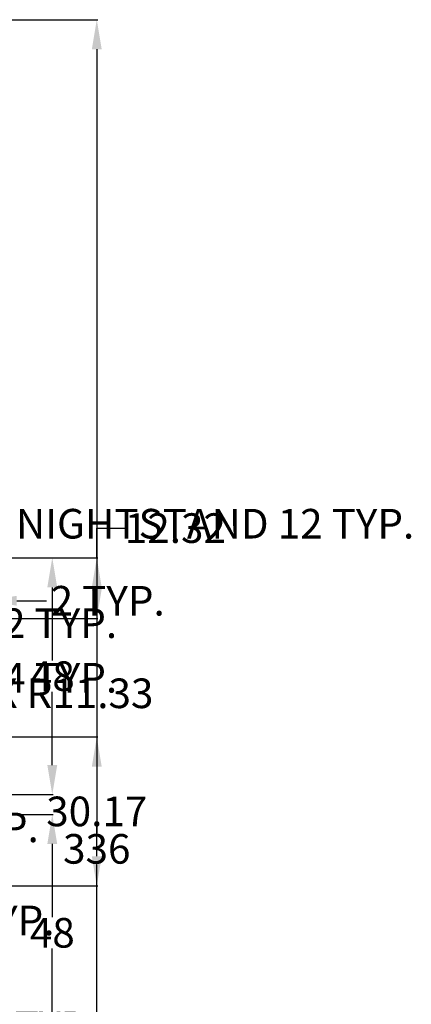
# Model space of a CAD drawing. Units: inches. Extents: x 98 to 487, y -240 to 141.
# Tile 5 of 5: x 408 to 487, y -81 to 119. Entities that reach past the tile are written whole.
import ezdxf

# ---------------------------------------------------------------- set-up
doc = ezdxf.new("R2010")
doc.units = ezdxf.units.IN
doc.header["$MEASUREMENT"] = 0
doc.layers.add('A-ANNO-DIMS', color=2, linetype='Continuous', lineweight=18)
doc.styles.get("Standard").update_dxf_attribs({"font": 'arial.ttf'})
doc.dimstyles.get("Standard").update_dxf_attribs({"dimtxt": 6, "dimasz": 6, "dimexe": 0.18, "dimexo": 0.0625, "dimgap": 0.09, "dimtad": 0, "dimtih": 1, "dimtoh": 1, "dimdec": 0, "dimzin": 0, "dimdsep": 46, "dimlunit": 4, "dimtxsty": 'Standard', "dimcen": 0.09, "dimadec": 0, "dimazin": 0, "dimtfac": 1, "dimtdec": 0, "dimtofl": 0, "dimtmove": 0, "dimatfit": 3, "dimfxl": 1, "dimtolj": 1, "dimtzin": 0, "dimarcsym": 0})

# ---------------------------------------------------------------- blocks, each defined once
blk = doc.blocks.new('*D26')
at = {"layer": 'A-ANNO-DIMS', "color": 0, "lineweight": -2, "transparency": 16777216}
for p, q in [((380.45, 18.25), (380.45, 16.33)), ((392.45, 18.25), (392.45, 16.33)), ((374.45, 16.51), (368.45, 16.51)), ((398.45, 16.51), (404.45, 16.51))]:
    blk.add_line(p, q, dxfattribs=at)
at = {"layer": 'A-ANNO-DIMS', "color": 0, "transparency": 16777216}
for points in [[(374.45, 17.51), (374.45, 15.51), (380.45, 16.51)], [(398.45, 17.51), (398.45, 15.51), (392.45, 16.51)]]:
    blk.add_solid(points, dxfattribs=at)
at = {"layer": 'Defpoints', "color": 0, "transparency": 16777216}
for p in [(380.45, 18.31), (392.45, 18.31), (392.45, 16.51)]:
    blk.add_point(p, dxfattribs=at)
at = {"layer": 'A-ANNO-DIMS', "color": 0, "transparency": 16777216, "insert": (447.4, 16.51), "char_height": 6, "attachment_point": 5}
blk.add_mtext('\\A1;NIGHTSTAND 12 TYP.', dxfattribs=at)
blk = doc.blocks.new('*D30')
at = {"layer": 'A-ANNO-DIMS', "color": 0, "lineweight": -2, "transparency": 16777216}
for p, q in [((399.2, -2.7), (395.49, -2.7)), ((395.67, -8.7), (395.67, -11.5)), ((395.67, -20.7), (395.67, -17.89)), ((399.2, -26.7), (395.49, -26.7))]:
    blk.add_line(p, q, dxfattribs=at)
at = {"layer": 'A-ANNO-DIMS', "color": 0, "transparency": 16777216}
for points in [[(394.67, -8.7), (396.67, -8.7), (395.67, -2.7)], [(394.67, -20.7), (396.67, -20.7), (395.67, -26.7)]]:
    blk.add_solid(points, dxfattribs=at)
at = {"layer": 'Defpoints', "color": 0, "transparency": 16777216}
for p in [(395.67, -2.7), (399.27, -2.7), (399.27, -26.7)]:
    blk.add_point(p, dxfattribs=at)
at = {"layer": 'A-ANNO-DIMS', "color": 0, "transparency": 16777216, "insert": (395.67, -14.7), "char_height": 6, "attachment_point": 5}
blk.add_mtext('\\A1;WINDOW 24 TYP.', dxfattribs=at)
blk = doc.blocks.new('*D31')
at = {"layer": 'A-ANNO-DIMS', "color": 0, "lineweight": -2, "transparency": 16777216}
for p, q in [((393.27, 0.9), (387.27, 0.9)), ((399.27, -2.64), (399.27, 1.08)), ((401.27, -2.64), (401.27, 1.08)), ((407.27, 0.9), (413.27, 0.9))]:
    blk.add_line(p, q, dxfattribs=at)
at = {"layer": 'A-ANNO-DIMS', "color": 0, "transparency": 16777216}
for points in [[(393.27, 1.9), (393.27, -0.1), (399.27, 0.9)], [(407.27, 1.9), (407.27, -0.1), (401.27, 0.9)]]:
    blk.add_solid(points, dxfattribs=at)
at = {"layer": 'Defpoints', "color": 0, "transparency": 16777216}
for p in [(401.27, 0.9), (399.27, -2.7), (401.27, -2.7)]:
    blk.add_point(p, dxfattribs=at)
at = {"layer": 'A-ANNO-DIMS', "color": 0, "transparency": 16777216, "insert": (425.68, 0.9), "char_height": 6, "attachment_point": 5}
blk.add_mtext('\\A1;2 TYP.', dxfattribs=at)
blk = doc.blocks.new('*D32')
at = {"layer": 'A-ANNO-DIMS', "color": 0, "lineweight": -2, "transparency": 16777216}
for p, q in [((348.74, -1.91), (348.74, -3.83)), ((360.78, -1.91), (360.78, -3.83)), ((342.74, -3.65), (336.74, -3.65)), ((366.78, -3.65), (372.78, -3.65))]:
    blk.add_line(p, q, dxfattribs=at)
at = {"layer": 'A-ANNO-DIMS', "color": 0, "transparency": 16777216}
for points in [[(342.74, -2.65), (342.74, -4.65), (348.74, -3.65)], [(366.78, -2.65), (366.78, -4.65), (360.78, -3.65)]]:
    blk.add_solid(points, dxfattribs=at)
at = {"layer": 'Defpoints', "color": 0, "transparency": 16777216}
for p in [(348.74, -1.85), (360.78, -1.85), (360.78, -3.65)]:
    blk.add_point(p, dxfattribs=at)
at = {"layer": 'A-ANNO-DIMS', "color": 0, "transparency": 16777216, "insert": (401.08, -3.65), "char_height": 6, "attachment_point": 5}
blk.add_mtext('\\A1;BASIN 12 TYP.', dxfattribs=at)
blk = doc.blocks.new('*D34')
at = {"layer": 'A-ANNO-DIMS', "color": 0, "lineweight": -2, "transparency": 16777216}
for p, q in [((347.1, -45.01), (341.1, -45.01)), ((353.1, -45.68), (353.1, -44.83)), ((358, -45.68), (358, -44.83)), ((364, -45.01), (370, -45.01))]:
    blk.add_line(p, q, dxfattribs=at)
at = {"layer": 'A-ANNO-DIMS', "color": 0, "transparency": 16777216}
for points in [[(347.1, -44.01), (347.1, -46.01), (353.1, -45.01)], [(364, -44.01), (364, -46.01), (358, -45.01)]]:
    blk.add_solid(points, dxfattribs=at)
at = {"layer": 'Defpoints', "color": 0, "transparency": 16777216}
for p in [(353.1, -45.75), (358, -45.01), (358, -45.75)]:
    blk.add_point(p, dxfattribs=at)
at = {"layer": 'A-ANNO-DIMS', "color": 0, "transparency": 16777216, "insert": (391.75, -45.01), "char_height": 6, "attachment_point": 5}
blk.add_mtext('\\A1;TAP 5 TYP.', dxfattribs=at)
blk = doc.blocks.new('*D36')
at = {"layer": 'A-ANNO-DIMS', "color": 0, "lineweight": -2, "transparency": 16777216}
for p, q in [((389.08, -47.36), (394.16, -47.36)), ((393.98, -53.36), (393.98, -60.69)), ((393.98, -74.4), (393.98, -67.08)), ((389.08, -80.4), (394.16, -80.4))]:
    blk.add_line(p, q, dxfattribs=at)
at = {"layer": 'A-ANNO-DIMS', "color": 0, "transparency": 16777216}
for points in [[(392.98, -53.36), (394.98, -53.36), (393.98, -47.36)], [(392.98, -74.4), (394.98, -74.4), (393.98, -80.4)]]:
    blk.add_solid(points, dxfattribs=at)
at = {"layer": 'Defpoints', "color": 0, "transparency": 16777216}
for p in [(389.02, -47.36), (393.98, -47.36), (389.02, -80.4)]:
    blk.add_point(p, dxfattribs=at)
at = {"layer": 'A-ANNO-DIMS', "color": 0, "transparency": 16777216, "insert": (393.98, -63.88), "char_height": 6, "attachment_point": 5}
blk.add_mtext('\\A1;WC 33 TYP.', dxfattribs=at)
blk = doc.blocks.new('*D37')
at = {"layer": 'A-ANNO-DIMS', "color": 0, "lineweight": -2, "transparency": 16777216}
for p, q in [((368.02, -80.47), (368.02, -85.54)), ((389.02, -80.47), (389.02, -85.54)), ((374.02, -85.36), (383.02, -85.36)), ((389.02, -85.36), (395.02, -85.36))]:
    blk.add_line(p, q, dxfattribs=at)
at = {"layer": 'A-ANNO-DIMS', "color": 0, "transparency": 16777216}
for points in [[(374.02, -84.36), (374.02, -86.36), (368.02, -85.36)], [(383.02, -84.36), (383.02, -86.36), (389.02, -85.36)]]:
    blk.add_solid(points, dxfattribs=at)
at = {"layer": 'Defpoints', "color": 0, "transparency": 16777216}
for p in [(368.02, -80.4), (389.02, -80.4), (389.02, -85.36)]:
    blk.add_point(p, dxfattribs=at)
at = {"layer": 'A-ANNO-DIMS', "color": 0, "transparency": 16777216, "insert": (409.76, -85.36), "char_height": 6, "attachment_point": 5}
blk.add_mtext('\\A1;21 TYP.', dxfattribs=at)
blk = doc.blocks.new('*D47')
at = {"layer": 'A-ANNO-DIMS', "color": 0, "lineweight": -2, "transparency": 16777216}
for p, q in [((404.83, 118.64), (423.65, 118.64)), ((423.47, 112.64), (423.47, -46.22)), ((423.47, -211.38), (423.47, -52.53)), ((404.83, -217.38), (423.65, -217.38))]:
    blk.add_line(p, q, dxfattribs=at)
at = {"layer": 'A-ANNO-DIMS', "color": 0, "transparency": 16777216}
for points in [[(422.47, 112.64), (424.47, 112.64), (423.47, 118.64)], [(422.47, -211.38), (424.47, -211.38), (423.47, -217.38)]]:
    blk.add_solid(points, dxfattribs=at)
at = {"layer": 'Defpoints', "color": 0, "transparency": 16777216}
for p in [(404.77, 118.64), (404.77, -217.38), (423.47, -217.38)]:
    blk.add_point(p, dxfattribs=at)
at = {"layer": 'A-ANNO-DIMS', "color": 0, "transparency": 16777216, "insert": (423.47, -49.37), "char_height": 6, "attachment_point": 5}
blk.add_mtext('\\A1;336', dxfattribs=at)
blk = doc.blocks.new('*D65')
at = {"layer": 'A-ANNO-DIMS', "color": 0, "lineweight": -2, "transparency": 16777216}
for p, q in [((395.83, 9.62), (414.65, 9.62)), ((414.47, 3.62), (414.47, -11.22)), ((414.47, -32.38), (414.47, -17.53)), ((395.83, -38.38), (414.65, -38.38))]:
    blk.add_line(p, q, dxfattribs=at)
at = {"layer": 'A-ANNO-DIMS', "color": 0, "transparency": 16777216}
for points in [[(413.47, 3.62), (415.47, 3.62), (414.47, 9.62)], [(413.47, -32.38), (415.47, -32.38), (414.47, -38.38)]]:
    blk.add_solid(points, dxfattribs=at)
at = {"layer": 'Defpoints', "color": 0, "transparency": 16777216}
for p in [(395.77, 9.62), (395.77, -38.38), (414.47, -38.38)]:
    blk.add_point(p, dxfattribs=at)
at = {"layer": 'A-ANNO-DIMS', "color": 0, "transparency": 16777216, "insert": (414.47, -14.38), "char_height": 6, "attachment_point": 5}
blk.add_mtext('\\A1;48', dxfattribs=at)
blk = doc.blocks.new('*D66')
at = {"layer": 'A-ANNO-DIMS', "color": 0, "lineweight": -2, "transparency": 16777216}
for p, q in [((395.83, -42.38), (414.65, -42.38)), ((414.47, -48.38), (414.47, -63.22)), ((414.47, -84.38), (414.47, -69.53)), ((395.83, -90.38), (414.65, -90.38))]:
    blk.add_line(p, q, dxfattribs=at)
at = {"layer": 'A-ANNO-DIMS', "color": 0, "transparency": 16777216}
for points in [[(413.47, -48.38), (415.47, -48.38), (414.47, -42.38)], [(413.47, -84.38), (415.47, -84.38), (414.47, -90.38)]]:
    blk.add_solid(points, dxfattribs=at)
at = {"layer": 'Defpoints', "color": 0, "transparency": 16777216}
for p in [(395.77, -42.38), (395.77, -90.38), (414.47, -90.38)]:
    blk.add_point(p, dxfattribs=at)
at = {"layer": 'A-ANNO-DIMS', "color": 0, "transparency": 16777216, "insert": (414.47, -66.38), "char_height": 6, "attachment_point": 5}
blk.add_mtext('\\A1;48', dxfattribs=at)
blk = doc.blocks.new('*D76')
at = {"layer": 'A-ANNO-DIMS', "color": 0, "lineweight": -2, "transparency": 16777216}
for p, q in [((404.83, -26.7), (423.65, -26.7)), ((423.47, -32.7), (423.47, -38.63)), ((423.47, -50.87), (423.47, -44.94)), ((404.83, -56.87), (423.65, -56.87))]:
    blk.add_line(p, q, dxfattribs=at)
at = {"layer": 'A-ANNO-DIMS', "color": 0, "transparency": 16777216}
for points in [[(422.47, -32.7), (424.47, -32.7), (423.47, -26.7)], [(422.47, -50.87), (424.47, -50.87), (423.47, -56.87)]]:
    blk.add_solid(points, dxfattribs=at)
at = {"layer": 'Defpoints', "color": 0, "transparency": 16777216}
for p in [(404.77, -26.7), (404.77, -56.87), (423.47, -56.87)]:
    blk.add_point(p, dxfattribs=at)
at = {"layer": 'A-ANNO-DIMS', "color": 0, "transparency": 16777216, "insert": (423.47, -41.78), "char_height": 6, "attachment_point": 5}
blk.add_mtext('\\A1;30.17', dxfattribs=at)
blk = doc.blocks.new('*D77')
at = {"layer": 'A-ANNO-DIMS', "color": 0, "lineweight": -2, "transparency": 16777216}
for p, q in [((423.47, 9.62), (423.47, 15.62)), ((423.47, 15.62), (429.47, 15.62)), ((395.83, 9.62), (423.65, 9.62)), ((423.47, 3.3), (423.47, 3.62)), ((404.83, -2.7), (423.65, -2.7))]:
    blk.add_line(p, q, dxfattribs=at)
at = {"layer": 'A-ANNO-DIMS', "color": 0, "transparency": 16777216}
for points in [[(422.47, 3.62), (424.47, 3.62), (423.47, 9.62)], [(422.47, 3.3), (424.47, 3.3), (423.47, -2.7)]]:
    blk.add_solid(points, dxfattribs=at)
at = {"layer": 'Defpoints', "color": 0, "transparency": 16777216}
for p in [(395.77, 9.62), (423.47, 9.62), (404.77, -2.7)]:
    blk.add_point(p, dxfattribs=at)
at = {"layer": 'A-ANNO-DIMS', "color": 0, "transparency": 16777216, "insert": (439.37, 15.62), "char_height": 6, "attachment_point": 5}
blk.add_mtext('\\A1;12.32', dxfattribs=at)
blk = doc.blocks.new('*D85')
at = {"layer": 'A-ANNO-DIMS', "color": 0, "lineweight": -2, "transparency": 16777216}
for p, q in [((373.71, -14.74), (373.89, -14.74)), ((373.8, -14.83), (373.8, -14.65)), ((396.92, -17.85), (390.97, -17.05))]:
    blk.add_line(p, q, dxfattribs=at)
at = {"layer": 'A-ANNO-DIMS', "color": 0, "transparency": 16777216}
blk.add_solid([(391.11, -16.06), (390.84, -18.04), (385.03, -16.25)], dxfattribs=at)
at = {"layer": 'Defpoints', "color": 0, "transparency": 16777216}
for p in [(373.8, -14.74), (385.03, -16.25)]:
    blk.add_point(p, dxfattribs=at)
at = {"layer": 'A-ANNO-DIMS', "color": 0, "transparency": 16777216, "insert": (416.57, -17.85), "char_height": 6, "attachment_point": 5}
blk.add_mtext('\\A1;4X R11.33', dxfattribs=at)

msp = doc.modelspace()

# ---------------------------------------------------------------- dimensions: what is measured, and where the dimension line sits
at = {"layer": 'A-ANNO-DIMS'}
for base, p1, p2, angle, override, picture, middle in [((423.4663, -217.3767), (404.7663, 118.6353), (404.7663, -217.3767), 90, {"dimdec": 0, "dimlfac": 1, "dimrnd": 0, "dimzin": 0, "dimdsep": 46, "dimlunit": 2}, '*D47', (423.4663, -49.3707)), ((423.4663, 9.6232), (404.7663, -2.698), (395.7663, 9.6232), 90, {"dimdec": 2, "dimlfac": 1, "dimrnd": 0, "dimzin": 0, "dimdsep": 46, "dimlunit": 2}, '*D77', (439.3667, 15.6232)), ((414.4663, -38.3769), (395.7663, 9.6232), (395.7663, -38.3769), 270, {"dimdec": 0, "dimlfac": 1, "dimrnd": 0, "dimzin": 0, "dimdsep": 46, "dimlunit": 2}, '*D65', (414.4663, -14.3768)), ((423.4663, -56.8658), (404.7663, -26.698), (404.7663, -56.8658), 90, {"dimdec": 2, "dimlfac": 1, "dimrnd": 0, "dimzin": 0, "dimdsep": 46, "dimlunit": 2}, '*D76', (423.4663, -41.7819)), ((414.4663, -90.3769), (395.7663, -42.3769), (395.7663, -90.3769), 270, {"dimdec": 0, "dimlfac": 1, "dimrnd": 0, "dimzin": 0, "dimdsep": 46, "dimlunit": 2}, '*D66', (414.4663, -66.3769))]:
    dim = msp.add_linear_dim(base=base, p1=p1, p2=p2, angle=angle, dimstyle='Standard', override=override, dxfattribs=at)
    dim.commit()
    dim.dimension.update_dxf_attribs({"geometry": picture, "text_midpoint": middle})
for base, p1, p2, text, picture, middle in [((392.4456, 16.5145), (380.4456, 18.3145), (392.4456, 18.3145), 'NIGHTSTAND <> TYP.', '*D26', (447.3992, 16.5145)), ((360.7769, -3.651), (348.7408, -1.8456), (360.7769, -1.8456), 'BASIN <> TYP.', '*D32', (401.0783, -3.651)), ((401.2663, 0.902), (399.2663, -2.698), (401.2663, -2.698), '<> TYP.', '*D31', (425.6796, 0.902)), ((357.9987, -45.012), (353.0963, -45.7474), (357.9987, -45.7474), 'TAP <> TYP.', '*D34', (391.7518, -45.012)), ((389.0194, -85.3611), (368.0194, -80.4041), (389.0194, -80.4041), '<> TYP.', '*D37', (409.7635, -85.3611))]:
    dim = msp.add_linear_dim(base=base, p1=p1, p2=p2, text=text, dimstyle='Standard', override={"dimdec": 0, "dimlfac": 1, "dimrnd": 0, "dimzin": 0, "dimdsep": 46, "dimlunit": 2}, dxfattribs=at)
    dim.commit()
    dim.dimension.update_dxf_attribs({"geometry": picture, "text_midpoint": middle})
for base, p1, p2, text, picture, middle in [((395.6663, -2.698), (399.2663, -26.698), (399.2663, -2.698), 'WINDOW <> TYP.', '*D30', (395.6663, -14.698)), ((393.9763, -47.3579), (389.0194, -80.4041), (389.0194, -47.3579), 'WC <> TYP.', '*D36', (393.9763, -63.881))]:
    dim = msp.add_linear_dim(base=base, p1=p1, p2=p2, angle=90, text=text, dimstyle='Standard', override={"dimdec": 0, "dimlfac": 1, "dimrnd": 0, "dimzin": 0, "dimdsep": 46, "dimlunit": 2}, dxfattribs=at)
    dim.commit()
    dim.dimension.update_dxf_attribs({"geometry": picture, "text_midpoint": middle})
dim = msp.add_radius_dim(center=(373.7984, -14.7446), mpoint=(385.0265, -16.2539), text='4X <>', dimstyle='Standard', override={"dimdec": 2, "dimlfac": 1, "dimrnd": 0, "dimzin": 0, "dimdsep": 46, "dimlunit": 2}, dxfattribs=at)
dim.commit()
dim.dimension.update_dxf_attribs({"geometry": '*D85', "text_midpoint": (416.571, -17.8526)})

doc.saveas('drawing.dxf')
